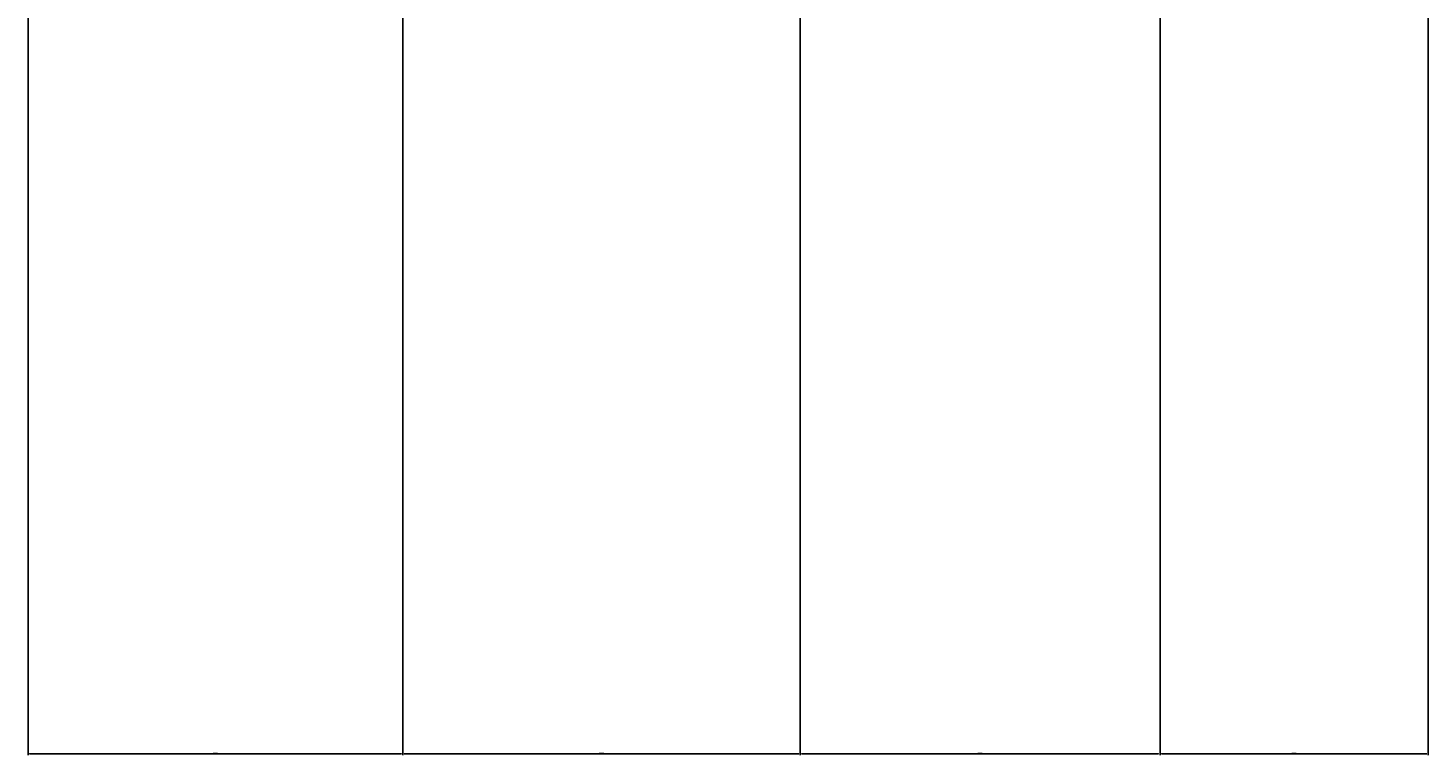
# Model space of a CAD drawing. Units: inches. Extents: x -301 to 715, y -607 to 364.
# Tile 130 of 141: x 310 to 497, y -607 to -510. Entities that reach past the tile are written whole.
import ezdxf

# ---------------------------------------------------------------- set-up
doc = ezdxf.new("R2010")
doc.units = ezdxf.units.IN
doc.header["$MEASUREMENT"] = 0
doc.layers.add('A-ANNO-DIMS', color=2, linetype='Continuous', lineweight=18)
doc.styles.get("Standard").update_dxf_attribs({"font": 'arial.ttf'})
doc.dimstyles.get("Standard").update_dxf_attribs({"dimtxt": 0.18, "dimasz": 0.18, "dimexe": 0.18, "dimexo": 0.0625, "dimgap": 0.09, "dimtad": 0, "dimtih": 1, "dimtoh": 1, "dimdec": 1, "dimzin": 0, "dimdsep": 46, "dimlunit": 4, "dimtxsty": 'Standard', "dimcen": 0.09, "dimclrd": 3, "dimclre": 4, "dimclrt": 6, "dimadec": 0, "dimazin": 0, "dimtfac": 1, "dimtdec": 1, "dimtofl": 0, "dimtmove": 0, "dimatfit": 3, "dimfxl": 1, "dimtfill": 2, "dimtfillclr": 51, "dimtolj": 1, "dimtzin": 0, "dimarcsym": 0})

# ---------------------------------------------------------------- blocks, each defined once
blk = doc.blocks.new('*D195')
at = {"layer": 'A-ANNO-DIMS', "color": 4, "lineweight": -2, "transparency": 16777216}
for p, q in [((310.02, -441.61), (310.02, -606.79)), ((360.02, -441.61), (360.02, -606.79))]:
    blk.add_line(p, q, dxfattribs=at)
at = {"layer": 'A-ANNO-DIMS', "color": 3, "lineweight": -2, "transparency": 16777216}
for p, q in [((310.2, -606.61), (334.68, -606.61)), ((359.84, -606.61), (335.35, -606.61))]:
    blk.add_line(p, q, dxfattribs=at)
at = {"layer": 'A-ANNO-DIMS', "color": 3, "transparency": 16777216}
for points in [[(310.2, -606.58), (310.2, -606.64), (310.02, -606.61)], [(359.84, -606.58), (359.84, -606.64), (360.02, -606.61)]]:
    blk.add_solid(points, dxfattribs=at)
at = {"layer": 'Defpoints', "color": 0, "transparency": 16777216}
for p in [(310.02, -441.55), (360.02, -441.55), (360.02, -606.61)]:
    blk.add_point(p, dxfattribs=at)
at = {"layer": 'A-ANNO-DIMS', "color": 6, "transparency": 16777216, "insert": (335.02, -606.61), "char_height": 0.18, "attachment_point": 5, "bg_fill": 1, "box_fill_scale": 1.25, "bg_fill_color": 51, "bg_fill_transparency": 0}
blk.add_mtext('\\A1;4\'-2"', dxfattribs=at)
blk = doc.blocks.new('*D196')
at = {"layer": 'A-ANNO-DIMS', "color": 4, "lineweight": -2, "transparency": 16777216}
for p, q in [((360.02, -441.61), (360.02, -606.79)), ((413.02, -489.61), (413.02, -606.79))]:
    blk.add_line(p, q, dxfattribs=at)
at = {"layer": 'A-ANNO-DIMS', "color": 3, "lineweight": -2, "transparency": 16777216}
for p, q in [((360.2, -606.61), (386.18, -606.61)), ((412.84, -606.61), (386.85, -606.61))]:
    blk.add_line(p, q, dxfattribs=at)
at = {"layer": 'A-ANNO-DIMS', "color": 3, "transparency": 16777216}
for points in [[(360.2, -606.58), (360.2, -606.64), (360.02, -606.61)], [(412.84, -606.58), (412.84, -606.64), (413.02, -606.61)]]:
    blk.add_solid(points, dxfattribs=at)
at = {"layer": 'Defpoints', "color": 0, "transparency": 16777216}
for p in [(360.02, -441.55), (413.02, -489.55), (413.02, -606.61)]:
    blk.add_point(p, dxfattribs=at)
at = {"layer": 'A-ANNO-DIMS', "color": 6, "transparency": 16777216, "insert": (386.52, -606.61), "char_height": 0.18, "attachment_point": 5, "bg_fill": 1, "box_fill_scale": 1.25, "bg_fill_color": 51, "bg_fill_transparency": 0}
blk.add_mtext('\\A1;4\'-5"', dxfattribs=at)
blk = doc.blocks.new('*D197')
at = {"layer": 'A-ANNO-DIMS', "color": 4, "lineweight": -2, "transparency": 16777216}
for p, q in [((413.02, -489.61), (413.02, -606.79)), ((461.02, -489.61), (461.02, -606.79))]:
    blk.add_line(p, q, dxfattribs=at)
at = {"layer": 'A-ANNO-DIMS', "color": 3, "lineweight": -2, "transparency": 16777216}
for p, q in [((413.2, -606.61), (436.68, -606.61)), ((460.84, -606.61), (437.35, -606.61))]:
    blk.add_line(p, q, dxfattribs=at)
at = {"layer": 'A-ANNO-DIMS', "color": 3, "transparency": 16777216}
for points in [[(413.2, -606.58), (413.2, -606.64), (413.02, -606.61)], [(460.84, -606.58), (460.84, -606.64), (461.02, -606.61)]]:
    blk.add_solid(points, dxfattribs=at)
at = {"layer": 'Defpoints', "color": 0, "transparency": 16777216}
for p in [(413.02, -489.55), (461.02, -489.55), (461.02, -606.61)]:
    blk.add_point(p, dxfattribs=at)
at = {"layer": 'A-ANNO-DIMS', "color": 6, "transparency": 16777216, "insert": (437.02, -606.61), "char_height": 0.18, "attachment_point": 5, "bg_fill": 1, "box_fill_scale": 1.25, "bg_fill_color": 51, "bg_fill_transparency": 0}
blk.add_mtext('\\A1;4\'-0"', dxfattribs=at)
blk = doc.blocks.new('*D198')
at = {"layer": 'A-ANNO-DIMS', "color": 4, "lineweight": -2, "transparency": 16777216}
for p, q in [((496.77, -441.61), (496.77, -606.79)), ((461.02, -489.61), (461.02, -606.79))]:
    blk.add_line(p, q, dxfattribs=at)
at = {"layer": 'A-ANNO-DIMS', "color": 3, "lineweight": -2, "transparency": 16777216}
for p, q in [((461.2, -606.61), (478.56, -606.61)), ((496.59, -606.61), (479.22, -606.61))]:
    blk.add_line(p, q, dxfattribs=at)
at = {"layer": 'A-ANNO-DIMS', "color": 3, "transparency": 16777216}
for points in [[(461.2, -606.58), (461.2, -606.64), (461.02, -606.61)], [(496.59, -606.58), (496.59, -606.64), (496.77, -606.61)]]:
    blk.add_solid(points, dxfattribs=at)
at = {"layer": 'Defpoints', "color": 0, "transparency": 16777216}
for p in [(496.77, -441.55), (461.02, -489.55), (496.77, -606.61)]:
    blk.add_point(p, dxfattribs=at)
at = {"layer": 'A-ANNO-DIMS', "color": 6, "transparency": 16777216, "insert": (478.89, -606.61), "char_height": 0.18, "attachment_point": 5, "bg_fill": 1, "box_fill_scale": 1.25, "bg_fill_color": 51, "bg_fill_transparency": 0}
blk.add_mtext('\\A1;3\'-0"', dxfattribs=at)

msp = doc.modelspace()

# ---------------------------------------------------------------- dimensions: what is measured, and where the dimension line sits
at = {"layer": 'A-ANNO-DIMS'}
for base, p1, p2, picture, middle in [((360.02, -606.61), (310.02, -441.55), (360.02, -441.55), '*D195', (335.02, -606.61)), ((413.02, -606.61), (360.02, -441.55), (413.02, -489.55), '*D196', (386.52, -606.61)), ((496.767813, -606.608725), (461.017813, -489.55247), (496.767813, -441.55247), '*D198', (478.892813, -606.608725)), ((461.02, -606.61), (413.02, -489.55), (461.02, -489.55), '*D197', (437.02, -606.61))]:
    dim = msp.add_linear_dim(base=base, p1=p1, p2=p2, dimstyle='Standard', override={"dimdec": 1, "dimlfac": 1, "dimrnd": 0, "dimzin": 1, "dimdsep": 46, "dimlunit": 4, "dimfrac": 2}, dxfattribs=at)
    dim.commit()
    dim.dimension.update_dxf_attribs({"geometry": picture, "text_midpoint": middle})

doc.saveas('drawing.dxf')
